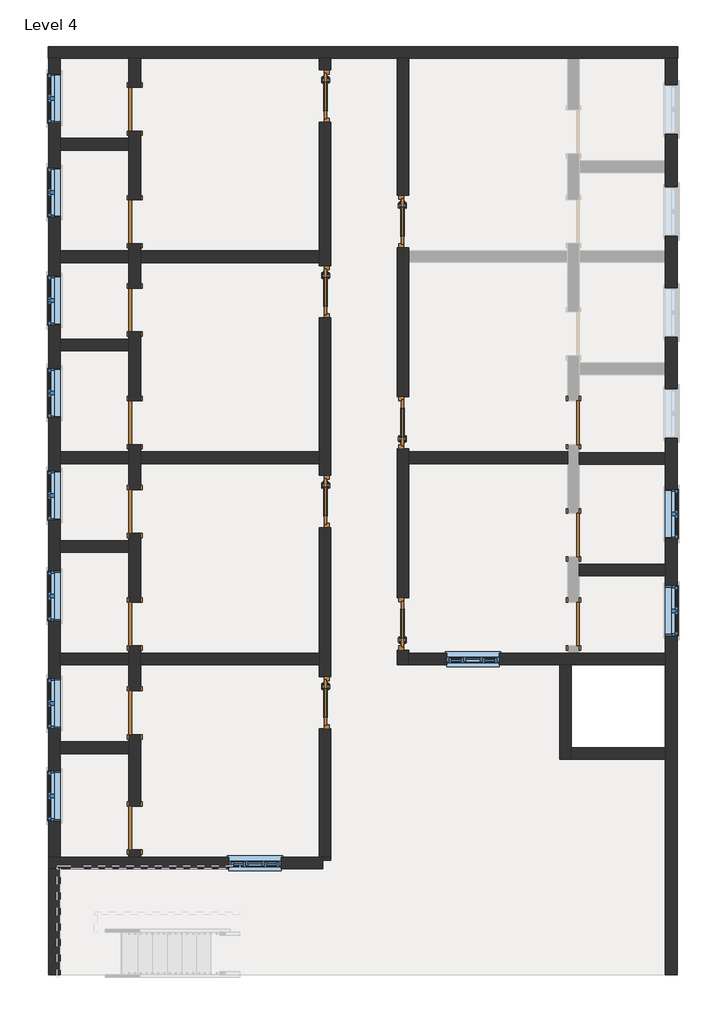
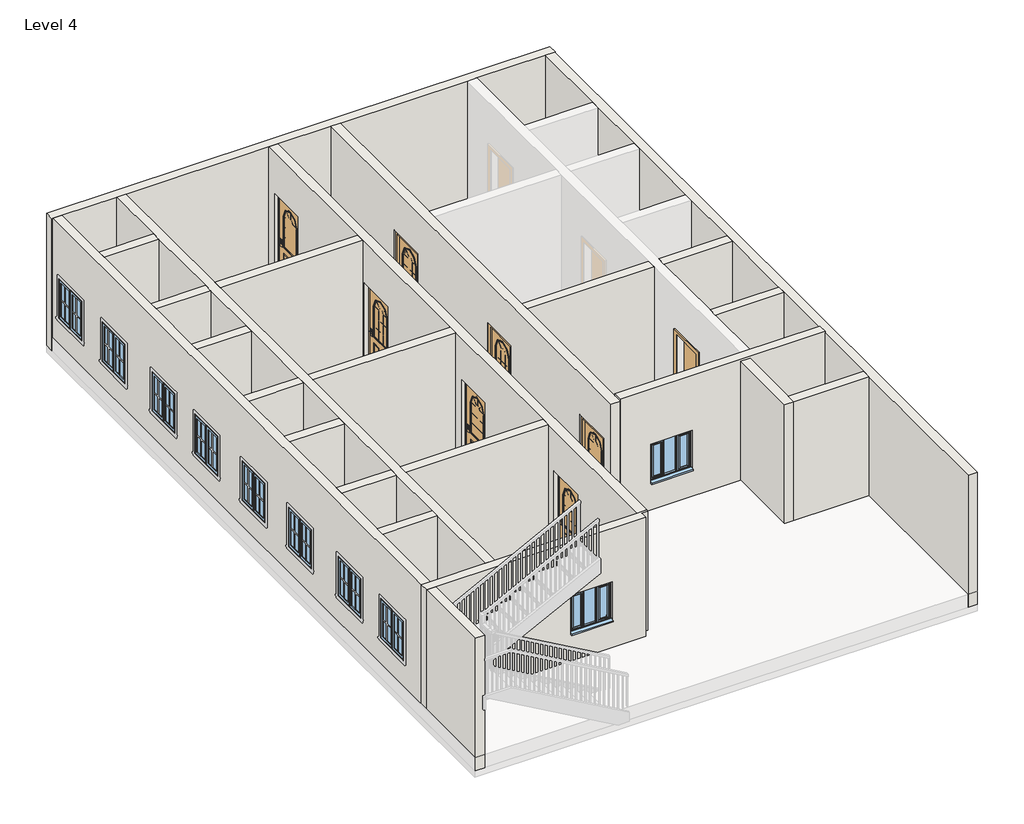
# One storey, part 1 of 4: 24 walls, 18 doors, 12 windows.
# Revit data of these elements (continued)
# Element 42 (IfcWall, "9\" w")
#   Top Offset = 0' - 0"
#   Base Offset = 0' - 0"
#   wall height = 10' - 0"
#   Phase Created = New Construction
#   Base Constraint = Level 4
#   Top Constraint = Level 5
#   Materials on its faces: "Default Wall", "Wood - Stained", "Earth"
# Element 43 (IfcWindow, "Window-Casement-Double : 34\" x 36\"")
#   Mark = "49"
#   Window Inset = 0' - 0"
#   Interior Wall Closure = 0' - 2 1/4"
#   Frame Extension = 0' - 0 1/4"
#   Exterior Wall Closure = 0' - 1 1/4"
#   Interior Trim Visibility = yes
#   Exterior Trim Visibility = yes
#   Phase Created = New Construction
#   Materials on its faces: "Wood - Stained", "Glass", "Clad - White"
# Element 44 (IfcWindow, "Window-Casement-Double : 34\" x 36\"")
#   Mark = "50"
#   Window Inset = 0' - 0"
#   Interior Wall Closure = 0' - 2 1/4"
#   Frame Extension = 0' - 0 1/4"
#   Exterior Wall Closure = 0' - 1 1/4"
#   Interior Trim Visibility = yes
#   Exterior Trim Visibility = yes
#   Phase Created = New Construction
#   Materials on its faces: "Wood - Stained", "Glass", "Clad - White"
# Element 45 (IfcWindow, "Window-Casement-Double : 34\" x 36\"")
#   Mark = "51"
#   Window Inset = 0' - 0"
#   Interior Wall Closure = 0' - 2 1/4"
#   Frame Extension = 0' - 0 1/4"
#   Exterior Wall Closure = 0' - 1 1/4"
#   Interior Trim Visibility = yes
#   Exterior Trim Visibility = yes
#   Phase Created = New Construction
#   Materials on its faces: "Wood - Stained", "Glass", "Clad - White"
# Element 46 (IfcWindow, "Window-Casement-Double : 34\" x 36\"")
#   Mark = "52"
#   Window Inset = 0' - 0"
#   Interior Wall Closure = 0' - 2 1/4"
#   Frame Extension = 0' - 0 1/4"
#   Exterior Wall Closure = 0' - 1 1/4"
#   Interior Trim Visibility = yes
#   Exterior Trim Visibility = yes
#   Phase Created = New Construction
#   Materials on its faces: "Wood - Stained", "Glass", "Clad - White"
# Element 47 (IfcWindow, "Window-Casement-Double : 34\" x 36\"")
#   Mark = "53"
#   Window Inset = 0' - 0"
#   Interior Wall Closure = 0' - 2 1/4"
#   Frame Extension = 0' - 0 1/4"
#   Exterior Wall Closure = 0' - 1 1/4"
#   Interior Trim Visibility = yes
#   Exterior Trim Visibility = yes
#   Phase Created = New Construction
#   Materials on its faces: "Wood - Stained", "Glass", "Clad - White"
# Element 48 (IfcWindow, "Window-Casement-Double : 34\" x 36\"")
#   Mark = "54"
#   Window Inset = 0' - 0"
#   Interior Wall Closure = 0' - 2 1/4"
#   Frame Extension = 0' - 0 1/4"
#   Exterior Wall Closure = 0' - 1 1/4"
#   Interior Trim Visibility = yes
#   Exterior Trim Visibility = yes
#   Phase Created = New Construction
#   Materials on its faces: "Wood - Stained", "Glass", "Clad - White"
# Element 49 (IfcWindow, "Window-Casement-Double : 34\" x 36\"")
#   Mark = "55"
#   Window Inset = 0' - 0"
#   Interior Wall Closure = 0' - 2 1/4"
#   Frame Extension = 0' - 0 1/4"
#   Exterior Wall Closure = 0' - 1 1/4"
#   Interior Trim Visibility = yes
#   Exterior Trim Visibility = yes
#   Phase Created = New Construction
#   Materials on its faces: "Wood - Stained", "Glass", "Clad - White"
# Element 50 (IfcWindow, "Window-Casement-Double : 34\" x 36\"")
#   Mark = "56"
#   Window Inset = 0' - 0"
#   Interior Wall Closure = 0' - 2 1/4"
#   Frame Extension = 0' - 0 1/4"
#   Exterior Wall Closure = 0' - 1 1/4"
#   Interior Trim Visibility = yes
#   Exterior Trim Visibility = yes
#   Phase Created = New Construction
#   Materials on its faces: "Wood - Stained", "Glass", "Clad - White"
# Element 51 (IfcWindow, "Window-Casement-Double : 34\" x 36\"")
#   Mark = "57"
#   Window Inset = 0' - 0"
#   Interior Wall Closure = 0' - 2 1/4"
#   Frame Extension = 0' - 0 1/4"
#   Exterior Wall Closure = 0' - 1 1/4"
#   Interior Trim Visibility = yes
#   Exterior Trim Visibility = yes
#   Phase Created = New Construction
#   Materials on its faces: "Wood - Stained", "Glass", "Clad - White"
# Element 52 (IfcWindow, "Window-Casement-Double : 34\" x 36\"")
#   Mark = "58"
#   Window Inset = 0' - 0"
#   Interior Wall Closure = 0' - 2 1/4"
#   Frame Extension = 0' - 0 1/4"
#   Exterior Wall Closure = 0' - 1 1/4"
#   Interior Trim Visibility = yes
#   Exterior Trim Visibility = yes
#   Phase Created = New Construction
#   Materials on its faces: "Wood - Stained", "Glass", "Clad - White"
# Element 53 (IfcWindow, "Windows_Tpl_Plain : 910x910mm")
#   Mark = "63"
#   Phase Created = New Construction
#   Materials on its faces: "Window Frame", "Glass"
# Element 54 (IfcWindow, "Windows_Tpl_Plain : 910x910mm")
#   Mark = "64"
#   Phase Created = New Construction
#   Materials on its faces: "Window Frame", "Glass"
# Materials
#   "Door - Glazing": colour RGB 0 0 255, transparency 0.75
#   "Door - Panel": class "Wood", colour RGB 210 159 95, transparency 0, Cost = 0
#   "Door - Frame/Mullion": class "Wood", colour RGB 212 179 113, transparency 0
#   "Door - Handle": colour RGB 247 247 247, transparency 0
#   "Door - Frame": colour RGB 118 70 51, transparency 0, Cost = 0
#   "Wood - Stained": class "Wood", colour RGB 224 178 126, transparency 0, Cost = 0
#   "Glass": class "Glass", colour RGB 0 128 192, transparency 0.75, Description = "Soda Lime Glass", Cost = 0
#   "Clad - White": class "Wood", colour RGB 242 242 238, transparency 0, Cost = 0
#   "Window Frame": colour RGB 249 249 249, transparency 0
#   "Default Wall": colour RGB 128 128 128, transparency 0, Cost = 0
#   "Brick, Common": class "Masonry", colour RGB 170 98 104, transparency 0, Description = "Common brick", Cost = 0
#   "Doors - Glazing Bars": colour RGB 158 107 65, transparency 0
#   "Cherry": class "Wood", colour RGB 226 177 128, transparency 0, Description = "Prunus Serotina", Cost = 0
#   "Earth": class "Generic", colour RGB 97 75 62, transparency 0, Description = "Soil", Cost = 0
